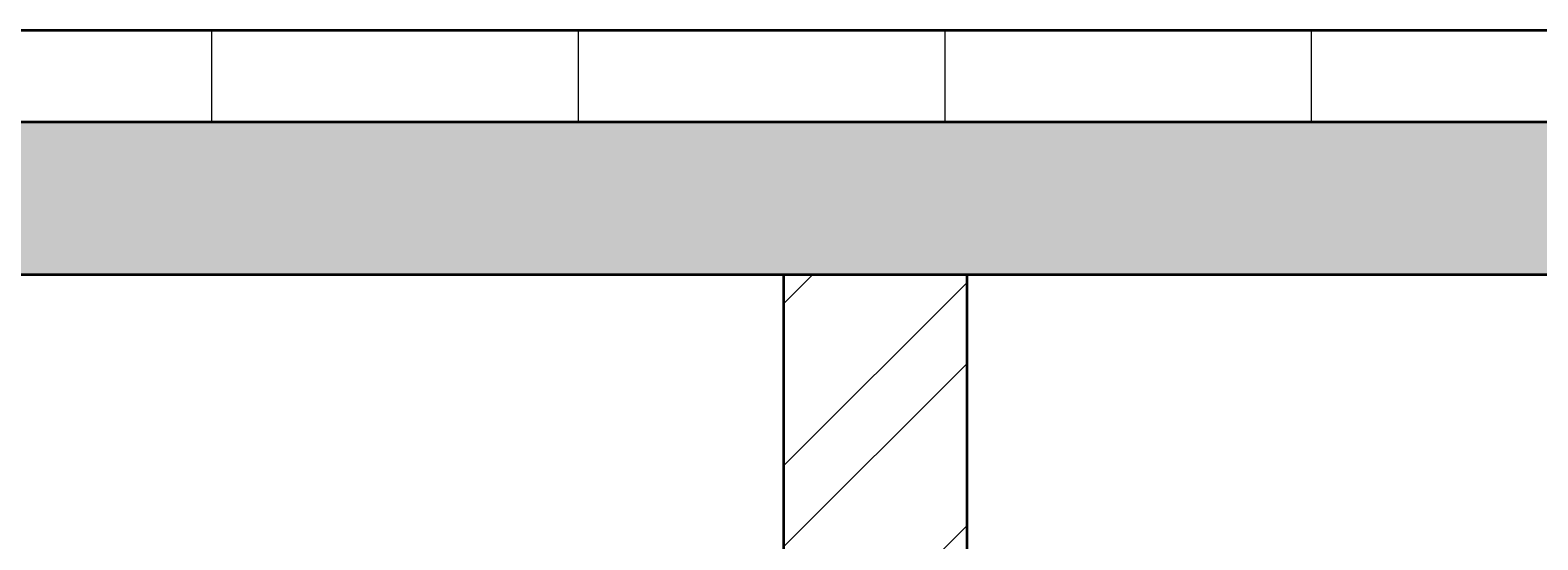
# Model space of a CAD drawing. Units: inches. Extents: x -301 to 715, y -607 to 364.
# Tile 42 of 141: x -66 to -17, y -370 to -353. Entities that reach past the tile are written whole.
import ezdxf

# ---------------------------------------------------------------- set-up
doc = ezdxf.new("R2010")
doc.units = ezdxf.units.IN
doc.header["$MEASUREMENT"] = 0
for name, color, linetype, lineweight in [('A-ANNO-DIMS', 2, 'Continuous', 18), ('A-SECT', 1, 'Continuous', 35), ('A-SECT-PATT', 8, 'Continuous', 13)]:
    doc.layers.add(name, color=color, linetype=linetype, lineweight=lineweight)
doc.styles.get("Standard").update_dxf_attribs({"font": 'arial.ttf'})
doc.dimstyles.get("Standard").update_dxf_attribs({"dimtxt": 0.18, "dimasz": 0.18, "dimexe": 0.18, "dimexo": 0.0625, "dimgap": 0.09, "dimtad": 0, "dimtih": 1, "dimtoh": 1, "dimdec": 1, "dimzin": 0, "dimdsep": 46, "dimlunit": 4, "dimtxsty": 'Standard', "dimcen": 0.09, "dimclrd": 3, "dimclre": 4, "dimclrt": 6, "dimadec": 0, "dimazin": 0, "dimtfac": 1, "dimtdec": 1, "dimtofl": 0, "dimtmove": 0, "dimatfit": 3, "dimfxl": 1, "dimtfill": 2, "dimtfillclr": 51, "dimtolj": 1, "dimtzin": 0, "dimarcsym": 0})

# ---------------------------------------------------------------- blocks, each defined once
blk = doc.blocks.new('*D189')
at = {"layer": 'A-ANNO-DIMS', "color": 4, "lineweight": -2, "transparency": 16777216}
for p, q in [((134.193, -353.477), (-266.112, -353.477)), ((134.193, -361.477), (-266.112, -361.477))]:
    blk.add_line(p, q, dxfattribs=at)
at = {"layer": 'A-ANNO-DIMS', "color": 3, "lineweight": -2, "transparency": 16777216}
for p, q in [((-265.932, -353.657), (-265.932, -357.296)), ((-265.932, -361.297), (-265.932, -357.659))]:
    blk.add_line(p, q, dxfattribs=at)
at = {"layer": 'A-ANNO-DIMS', "color": 3, "transparency": 16777216}
for points in [[(-265.962, -353.657), (-265.902, -353.657), (-265.932, -353.477)], [(-265.962, -361.297), (-265.902, -361.297), (-265.932, -361.477)]]:
    blk.add_solid(points, dxfattribs=at)
at = {"layer": 'Defpoints', "color": 0, "transparency": 16777216}
for p in [(134.255, -353.477), (-265.932, -361.477), (134.255, -361.477)]:
    blk.add_point(p, dxfattribs=at)
at = {"layer": 'A-ANNO-DIMS', "color": 6, "transparency": 16777216, "insert": (-265.932, -357.477), "char_height": 0.18, "attachment_point": 5, "bg_fill": 1, "box_fill_scale": 1.25, "bg_fill_color": 51, "bg_fill_transparency": 0}
blk.add_mtext('\\A1;0\'-8"', dxfattribs=at)

msp = doc.modelspace()

# ---------------------------------------------------------------- hatches: boundary and pattern name
at = {"layer": 'A-SECT-PATT'}
h = msp.add_hatch(dxfattribs=at)
h.set_pattern_fill('ANSI31', color=256, scale=96, angle=45, style=0)
h.paths.add_polyline_path([(-185.282, -356.477), (134.255, -356.477), (134.255, -353.477), (-185.282, -353.477)])
h = msp.add_hatch(dxfattribs=at)
h.set_pattern_fill('AR-CONC', color=256, scale=0.5)
h.set_pattern_definition([(50, (10.3213, 33.8764), (3.586301, -0.31376), [0.375, -4.125]), (355, (10.3213, 33.8764), (-0.693757, 3.76096), [0.3, -3.3]), (100.45144, (10.62, 33.8502), (2.892544, 3.4472), [0.3187, -3.50571]), (46.1842, (10.3213, 34.8764), (5.336207, -0.827596), [0.5625, -6.1875]), (96.6356, (10.766, 34.8074), (4.67331, 4.870593), [0.47805, -5.25857]), (351.1842, (10.321, 34.8764), (4.67331, 4.870593), [0.45, -4.95]), (21, (10.8213, 34.6264), (2.984535, -2.013094), [0.375, -4.125]), (326, (10.8213, 34.6264), (1.216577, 3.62575), [0.3, -3.3]), (71.45144, (11.07, 34.4586), (4.201112, 1.612656), [0.3187, -3.50571]), (37.5, (10.3213, 33.8764), (0.0607993, 1.6644693), [0, -3.26, 0, -3.35, 0, -3.3125]), (7.5, (10.3213, 33.8764), (1.3153477, 1.9720586), [0, -1.91, 0, -3.185, 0, -1.2625]), (327.5, (9.2063, 33.8764), (2.6691122, -0.1127744), [0, -1.25, 0, -3.9, 0, -5.175]), (317.5, (8.7063, 33.8764), (2.915931, 0.500525), [0, -1.625, 0, -2.59, 0, -3.675])])
h.paths.add_polyline_path([(-56.282, -535.477), (-61.282, -535.477), (-61.282, -540.477), (-15.282, -540.477), (-15.282, -535.477), (-20.282, -535.477)])
h.paths.add_polyline_path([(119.255, -535.477), (114.255, -535.477), (114.255, -540.477), (163.255, -540.477), (163.255, -535.477), (158.255, -535.477)])
h.paths.add_polyline_path([(-206.282, -471.477), (-209.282, -471.477), (-209.282, -481.477), (-206.282, -481.477), (-194.282, -481.477), (-194.282, -471.477)])
h.paths.add_polyline_path([(-41.282, -481.477), (-41.282, -471.477), (-185.282, -471.477), (-185.282, -481.477), (-180.282, -481.477)])
h.paths.add_polyline_path([(134.255, -481.477), (134.255, -471.477), (-35.282, -471.477), (-35.282, -481.477), (-30.282, -481.477)])
h.paths.add_polyline_path([(155.218, -481.477), (158.218, -481.477), (158.218, -471.477), (153.218, -471.477), (143.218, -471.477), (143.218, -481.477), (148.255, -481.477)])
h.paths.add_polyline_path([(-193.88, -356.477), (-193.904, -361.477), (143.218, -361.477), (143.218, -356.477)])
h = msp.add_hatch(dxfattribs=at)
h.set_pattern_fill('ANSI32', color=256, scale=15)
h.set_pattern_definition([(45, (10.321, 33.8764), (-3.977476, 3.977476), []), (45, (12.973, 33.8764), (-3.977476, 3.977476), [])])
h.paths.add_polyline_path([(-35.282, -361.477), (-41.282, -361.477), (-41.282, -376.452), (-35.282, -376.452)])
h.paths.add_polyline_path([(143.218, -439.477), (134.255, -439.477), (134.255, -463.477), (143.218, -463.477)])

# ---------------------------------------------------------------- linework, layer by layer
at = {"layer": 'A-SECT'}
for p, q in [((-194.282, -353.477), (143.218, -353.477)), ((-194.282, -356.477), (143.218, -356.477)), ((-194.282, -361.477), (143.218, -361.477)), ((-41.282, -361.477), (-41.282, -481.477)), ((-35.282, -361.477), (-35.282, -463.477))]:
    msp.add_line(p, q, dxfattribs=at)

# ---------------------------------------------------------------- dimensions: what is measured, and where the dimension line sits
at = {"layer": 'A-ANNO-DIMS'}
dim = msp.add_linear_dim(base=(-265.932, -361.477), p1=(134.255, -353.477), p2=(134.255, -361.477), angle=90, dimstyle='Standard', override={"dimdec": 1, "dimlfac": 1, "dimrnd": 0, "dimzin": 1, "dimdsep": 46, "dimlunit": 4, "dimfrac": 2}, dxfattribs=at)
dim.commit()
dim.dimension.update_dxf_attribs({"geometry": '*D189', "text_midpoint": (-265.932, -357.477)})

doc.saveas('drawing.dxf')
